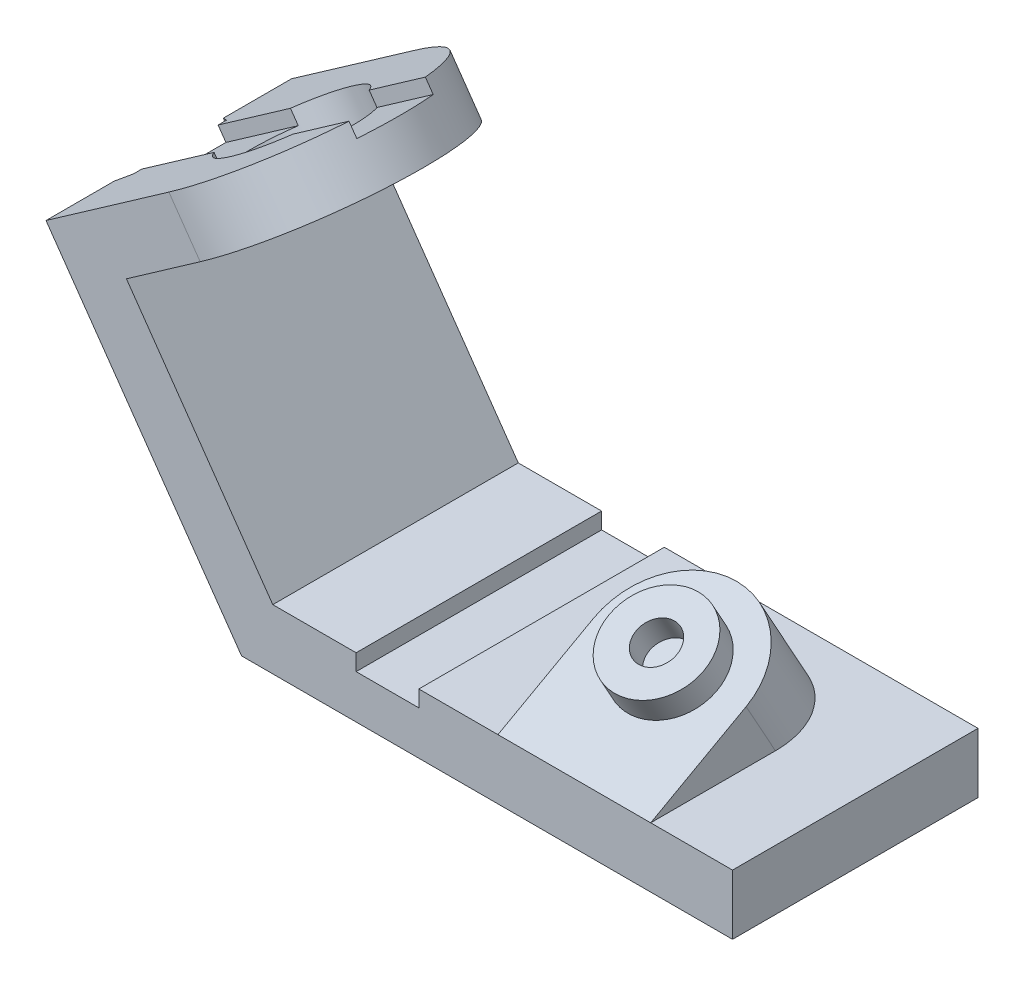
ISO-10303-21;
HEADER;
FILE_DESCRIPTION(('STEP AP214'),'2;1');
FILE_NAME('part.step','',(''),(''),'','','');
FILE_SCHEMA(('AUTOMOTIVE_DESIGN { 1 0 10303 214 1 1 1 1 }'));
ENDSEC;
DATA;
#1=APPLICATION_CONTEXT('core data for automotive mechanical design processes');
#2=APPLICATION_PROTOCOL_DEFINITION('international standard','automotive_design',2000,#1);
#3=PRODUCT_CONTEXT('',#1,'mechanical');
#4=PRODUCT('Part','Part','',(#3));
#5=PRODUCT_RELATED_PRODUCT_CATEGORY('part','',(#4));
#6=PRODUCT_DEFINITION_FORMATION('','',#4);
#7=PRODUCT_DEFINITION_CONTEXT('part definition',#1,'design');
#8=PRODUCT_DEFINITION('design','',#6,#7);
#9=PRODUCT_DEFINITION_SHAPE('','',#8);
#10=(LENGTH_UNIT() NAMED_UNIT(*) SI_UNIT(.MILLI.,.METRE.));
#11=(NAMED_UNIT(*) PLANE_ANGLE_UNIT() SI_UNIT($,.RADIAN.));
#12=(NAMED_UNIT(*) SI_UNIT($,.STERADIAN.) SOLID_ANGLE_UNIT());
#13=UNCERTAINTY_MEASURE_WITH_UNIT(LENGTH_MEASURE(1.E-05),#10,'distance_accuracy_value','');
#14=(GEOMETRIC_REPRESENTATION_CONTEXT(3) GLOBAL_UNCERTAINTY_ASSIGNED_CONTEXT((#13)) GLOBAL_UNIT_ASSIGNED_CONTEXT((#10,
#11,#12)) REPRESENTATION_CONTEXT('',''));
#15=CARTESIAN_POINT('',(0.,0.,0.));
#16=DIRECTION('',(0.,0.,1.));
#17=DIRECTION('',(1.,0.,0.));
#18=AXIS2_PLACEMENT_3D('',#15,#16,#17);
#19=CARTESIAN_POINT('',(-143.675709569523,115.012687135847,45.));
#20=DIRECTION('',(0.573576436351044,-0.819152044288993,0.));
#21=DIRECTION('',(0.819152044288993,0.573576436351044,0.));
#22=AXIS2_PLACEMENT_3D('',#19,#20,#21);
#23=PLANE('',#22);
#24=DIRECTION('',(0.,0.,-1.));
#25=VECTOR('',#24,1.);
#26=CARTESIAN_POINT('',(-157.601294322436,105.261887717879,-17.1132486540519));
#27=LINE('',#26,#25);
#28=CARTESIAN_POINT('',(-157.601294322436,105.261887717879,-14.));
#29=VERTEX_POINT('',#28);
#30=CARTESIAN_POINT('',(-157.601294322436,105.261887717879,-17.1132486540519));
#31=VERTEX_POINT('',#30);
#32=EDGE_CURVE('E277',#29,#31,#27,.T.);
#33=ORIENTED_EDGE('',*,*,#32,.F.);
#34=DIRECTION('',(-0.819152044288993,-0.573576436351044,0.));
#35=VECTOR('',#34,1.);
#36=CARTESIAN_POINT('',(-157.601294322436,105.261887717879,-14.));
#37=LINE('',#36,#35);
#38=CARTESIAN_POINT('',(-131.072166550331,123.837782966036,-14.));
#39=VERTEX_POINT('',#38);
#40=EDGE_CURVE('E236',#39,#29,#37,.T.);
#41=ORIENTED_EDGE('',*,*,#40,.F.);
#42=CARTESIAN_POINT('',(-116.643692107986,133.940709535432,0.));
#43=DIRECTION('',(-0.573576436351044,0.819152044288993,0.));
#44=DIRECTION('',(-0.819152044288993,-0.573576436351044,0.));
#45=AXIS2_PLACEMENT_3D('',#42,#43,#44);
#46=CIRCLE('',#45,22.5);
#47=CARTESIAN_POINT('',(-102.215217665641,144.043636104827,-14.));
#48=VERTEX_POINT('',#47);
#49=EDGE_CURVE('E292',#48,#39,#46,.T.);
#50=ORIENTED_EDGE('',*,*,#49,.F.);
#51=DIRECTION('',(-0.819152044288993,-0.573576436351044,0.));
#52=VECTOR('',#51,1.);
#53=CARTESIAN_POINT('',(-102.215217665641,144.043636104827,-14.));
#54=LINE('',#53,#52);
#55=CARTESIAN_POINT('',(-81.6111726286317,158.470743757354,-14.));
#56=VERTEX_POINT('',#55);
#57=EDGE_CURVE('E255',#56,#48,#54,.T.);
#58=ORIENTED_EDGE('',*,*,#57,.F.);
#59=CARTESIAN_POINT('',(-116.643692107986,133.940709535432,0.));
#60=DIRECTION('',(-0.573576436351044,0.819152044288993,0.));
#61=DIRECTION('',(-0.819152044288993,-0.573576436351044,0.));
#62=AXIS2_PLACEMENT_3D('',#59,#60,#61);
#63=CIRCLE('',#62,45.);
#64=CARTESIAN_POINT('',(-116.643692107986,133.940709535432,-45.));
#65=VERTEX_POINT('',#64);
#66=EDGE_CURVE('E314',#56,#65,#63,.T.);
#67=ORIENTED_EDGE('',*,*,#66,.T.);
#68=DIRECTION('',(-0.819152044288993,-0.573576436351044,0.));
#69=VECTOR('',#68,1.);
#70=CARTESIAN_POINT('',(-143.675709569523,115.012687135847,-45.));
#71=LINE('',#70,#69);
#72=CARTESIAN_POINT('',(-161.697054543881,102.394005536124,-45.));
#73=VERTEX_POINT('',#72);
#74=EDGE_CURVE('E336',#65,#73,#71,.T.);
#75=ORIENTED_EDGE('',*,*,#74,.T.);
#76=DIRECTION('',(0.,0.,1.));
#77=VECTOR('',#76,1.);
#78=CARTESIAN_POINT('',(-161.697054543881,102.394005536124,45.));
#79=LINE('',#78,#77);
#80=CARTESIAN_POINT('',(-161.697054543881,102.394005536124,-20.));
#81=VERTEX_POINT('',#80);
#82=EDGE_CURVE('E330',#73,#81,#79,.T.);
#83=ORIENTED_EDGE('',*,*,#82,.T.);
#84=DIRECTION('',(-0.709406479916225,-0.49673176489215,-0.500000000000001));
#85=VECTOR('',#84,1.);
#86=CARTESIAN_POINT('',(-161.697054543881,102.394005536124,-20.));
#87=LINE('',#86,#85);
#88=EDGE_CURVE('E279',#31,#81,#87,.T.);
#89=ORIENTED_EDGE('',*,*,#88,.F.);
#90=EDGE_LOOP('',(#33,#41,#50,#58,#67,#75,#83,#89));
#91=FACE_BOUND('',#90,.T.);
#92=ADVANCED_FACE('F44',(#91),#23,.F.);
#93=CARTESIAN_POINT('',(-60.3909064496553,-42.2861679353658,0.));
#94=DIRECTION('',(-0.819152044288993,-0.573576436351044,0.));
#95=DIRECTION('',(0.573576436351044,-0.819152044288993,0.));
#96=AXIS2_PLACEMENT_3D('',#93,#94,#95);
#97=PLANE('',#96);
#98=DIRECTION('',(0.573576436351044,-0.819152044288993,0.));
#99=VECTOR('',#98,1.);
#100=CARTESIAN_POINT('',(-60.3909064496553,-42.2861679353658,-20.));
#101=LINE('',#100,#99);
#102=CARTESIAN_POINT('',(-90.,0.,-20.));
#103=VERTEX_POINT('',#102);
#104=EDGE_CURVE('E52',#81,#103,#101,.T.);
#105=ORIENTED_EDGE('',*,*,#104,.F.);
#106=ORIENTED_EDGE('',*,*,#82,.F.);
#107=DIRECTION('',(-0.573576436351044,0.819152044288993,0.));
#108=VECTOR('',#107,1.);
#109=CARTESIAN_POINT('',(-90.,0.,-45.));
#110=LINE('',#109,#108);
#111=CARTESIAN_POINT('',(-90.,0.,-45.));
#112=VERTEX_POINT('',#111);
#113=EDGE_CURVE('E335',#112,#73,#110,.T.);
#114=ORIENTED_EDGE('',*,*,#113,.F.);
#115=DIRECTION('',(0.,0.,1.));
#116=VECTOR('',#115,1.);
#117=CARTESIAN_POINT('',(-90.,0.,45.));
#118=LINE('',#117,#116);
#119=EDGE_CURVE('E422',#112,#103,#118,.T.);
#120=ORIENTED_EDGE('',*,*,#119,.T.);
#121=EDGE_LOOP('',(#105,#106,#114,#120));
#122=FACE_BOUND('',#121,.T.);
#123=ADVANCED_FACE('F454',(#122),#97,.T.);
#124=CARTESIAN_POINT('',(-42.3695614752975,-29.6674863356428,0.));
#125=DIRECTION('',(-0.819152044288993,-0.573576436351044,0.));
#126=DIRECTION('',(0.573576436351044,-0.819152044288993,0.));
#127=AXIS2_PLACEMENT_3D('',#124,#125,#126);
#128=PLANE('',#127);
#129=DIRECTION('',(0.,0.,-1.));
#130=VECTOR('',#129,1.);
#131=CARTESIAN_POINT('',(-132.204180842502,98.6296462500672,0.));
#132=LINE('',#131,#130);
#133=CARTESIAN_POINT('',(-132.204180842502,98.6296462500672,45.));
#134=VERTEX_POINT('',#133);
#135=CARTESIAN_POINT('',(-132.204180842502,98.6296462500672,-45.));
#136=VERTEX_POINT('',#135);
#137=EDGE_CURVE('E318',#134,#136,#132,.T.);
#138=ORIENTED_EDGE('',*,*,#137,.F.);
#139=DIRECTION('',(0.573576436351044,-0.819152044288993,0.));
#140=VECTOR('',#139,1.);
#141=CARTESIAN_POINT('',(-71.9786550256421,12.618681599723,45.));
#142=LINE('',#141,#140);
#143=CARTESIAN_POINT('',(-78.5475248878616,22.,45.));
#144=VERTEX_POINT('',#143);
#145=EDGE_CURVE('E322',#134,#144,#142,.T.);
#146=ORIENTED_EDGE('',*,*,#145,.T.);
#147=DIRECTION('',(0.,0.,-1.));
#148=VECTOR('',#147,1.);
#149=CARTESIAN_POINT('',(-78.5475248878616,22.,0.));
#150=LINE('',#149,#148);
#151=CARTESIAN_POINT('',(-78.5475248878616,22.,-45.));
#152=VERTEX_POINT('',#151);
#153=EDGE_CURVE('E345',#144,#152,#150,.T.);
#154=ORIENTED_EDGE('',*,*,#153,.T.);
#155=DIRECTION('',(-0.573576436351044,0.819152044288993,0.));
#156=VECTOR('',#155,1.);
#157=CARTESIAN_POINT('',(-71.9786550256421,12.618681599723,-45.));
#158=LINE('',#157,#156);
#159=EDGE_CURVE('E326',#152,#136,#158,.T.);
#160=ORIENTED_EDGE('',*,*,#159,.T.);
#161=EDGE_LOOP('',(#138,#146,#154,#160));
#162=FACE_BOUND('',#161,.T.);
#163=ADVANCED_FACE('F474',(#162),#128,.F.);
#164=CARTESIAN_POINT('',(0.,22.,0.));
#165=DIRECTION('',(0.,-1.,0.));
#166=DIRECTION('',(0.,0.,-1.));
#167=AXIS2_PLACEMENT_3D('',#164,#165,#166);
#168=PLANE('',#167);
#169=ORIENTED_EDGE('',*,*,#153,.F.);
#170=DIRECTION('',(1.,0.,0.));
#171=VECTOR('',#170,1.);
#172=CARTESIAN_POINT('',(-90.,22.,45.));
#173=LINE('',#172,#171);
#174=CARTESIAN_POINT('',(-48.,22.,45.));
#175=VERTEX_POINT('',#174);
#176=EDGE_CURVE('E418',#144,#175,#173,.T.);
#177=ORIENTED_EDGE('',*,*,#176,.T.);
#178=DIRECTION('',(0.,0.,1.));
#179=VECTOR('',#178,1.);
#180=CARTESIAN_POINT('',(-48.,22.,-45.));
#181=LINE('',#180,#179);
#182=CARTESIAN_POINT('',(-48.,22.,-45.));
#183=VERTEX_POINT('',#182);
#184=EDGE_CURVE('E341',#183,#175,#181,.T.);
#185=ORIENTED_EDGE('',*,*,#184,.F.);
#186=DIRECTION('',(-1.,0.,0.));
#187=VECTOR('',#186,1.);
#188=CARTESIAN_POINT('',(-90.,22.,-45.));
#189=LINE('',#188,#187);
#190=EDGE_CURVE('E408',#183,#152,#189,.T.);
#191=ORIENTED_EDGE('',*,*,#190,.T.);
#192=EDGE_LOOP('',(#169,#177,#185,#191));
#193=FACE_BOUND('',#192,.T.);
#194=ADVANCED_FACE('F483',(#193),#168,.F.);
#195=CARTESIAN_POINT('',(90.,22.,45.));
#196=DIRECTION('',(-1.,0.,0.));
#197=DIRECTION('',(0.,0.,1.));
#198=AXIS2_PLACEMENT_3D('',#195,#196,#197);
#199=PLANE('',#198);
#200=DIRECTION('',(0.,0.,-1.));
#201=VECTOR('',#200,1.);
#202=CARTESIAN_POINT('',(90.,0.,45.));
#203=LINE('',#202,#201);
#204=CARTESIAN_POINT('',(90.,0.,45.));
#205=VERTEX_POINT('',#204);
#206=CARTESIAN_POINT('',(90.,0.,-45.));
#207=VERTEX_POINT('',#206);
#208=EDGE_CURVE('E394',#205,#207,#203,.T.);
#209=ORIENTED_EDGE('',*,*,#208,.T.);
#210=DIRECTION('',(0.,-1.,0.));
#211=VECTOR('',#210,1.);
#212=CARTESIAN_POINT('',(90.,22.,-45.));
#213=LINE('',#212,#211);
#214=CARTESIAN_POINT('',(90.,22.,-45.));
#215=VERTEX_POINT('',#214);
#216=EDGE_CURVE('E431',#215,#207,#213,.T.);
#217=ORIENTED_EDGE('',*,*,#216,.F.);
#218=DIRECTION('',(0.,0.,-1.));
#219=VECTOR('',#218,1.);
#220=CARTESIAN_POINT('',(90.,22.,45.));
#221=LINE('',#220,#219);
#222=CARTESIAN_POINT('',(90.,22.,45.));
#223=VERTEX_POINT('',#222);
#224=EDGE_CURVE('E409',#223,#215,#221,.T.);
#225=ORIENTED_EDGE('',*,*,#224,.F.);
#226=DIRECTION('',(0.,-1.,0.));
#227=VECTOR('',#226,1.);
#228=CARTESIAN_POINT('',(90.,22.,45.));
#229=LINE('',#228,#227);
#230=EDGE_CURVE('E416',#223,#205,#229,.T.);
#231=ORIENTED_EDGE('',*,*,#230,.T.);
#232=EDGE_LOOP('',(#209,#217,#225,#231));
#233=FACE_BOUND('',#232,.T.);
#234=ADVANCED_FACE('F50',(#233),#199,.F.);
#235=CARTESIAN_POINT('',(-90.,22.,-45.));
#236=DIRECTION('',(0.,0.,1.));
#237=DIRECTION('',(1.,0.,0.));
#238=AXIS2_PLACEMENT_3D('',#235,#236,#237);
#239=PLANE('',#238);
#240=ORIENTED_EDGE('',*,*,#74,.F.);
#241=DIRECTION('',(-0.573576436351044,0.819152044288993,0.));
#242=VECTOR('',#241,1.);
#243=CARTESIAN_POINT('',(-105.172163380965,117.557668649652,-45.));
#244=LINE('',#243,#242);
#245=CARTESIAN_POINT('',(-105.172163380965,117.557668649652,-45.));
#246=VERTEX_POINT('',#245);
#247=EDGE_CURVE('E313',#246,#65,#244,.T.);
#248=ORIENTED_EDGE('',*,*,#247,.F.);
#249=DIRECTION('',(-0.819152044288993,-0.573576436351044,0.));
#250=VECTOR('',#249,1.);
#251=CARTESIAN_POINT('',(-105.172163380965,117.557668649652,-45.));
#252=LINE('',#251,#250);
#253=EDGE_CURVE('E301',#246,#136,#252,.T.);
#254=ORIENTED_EDGE('',*,*,#253,.T.);
#255=ORIENTED_EDGE('',*,*,#159,.F.);
#256=ORIENTED_EDGE('',*,*,#190,.F.);
#257=DIRECTION('',(0.,1.,0.));
#258=VECTOR('',#257,1.);
#259=CARTESIAN_POINT('',(-48.,16.,-45.));
#260=LINE('',#259,#258);
#261=CARTESIAN_POINT('',(-48.,16.,-45.));
#262=VERTEX_POINT('',#261);
#263=EDGE_CURVE('E361',#262,#183,#260,.T.);
#264=ORIENTED_EDGE('',*,*,#263,.F.);
#265=DIRECTION('',(-1.,0.,0.));
#266=VECTOR('',#265,1.);
#267=CARTESIAN_POINT('',(-48.,16.,-45.));
#268=LINE('',#267,#266);
#269=CARTESIAN_POINT('',(-25.,16.,-45.));
#270=VERTEX_POINT('',#269);
#271=EDGE_CURVE('E357',#270,#262,#268,.T.);
#272=ORIENTED_EDGE('',*,*,#271,.F.);
#273=DIRECTION('',(0.,1.,0.));
#274=VECTOR('',#273,1.);
#275=CARTESIAN_POINT('',(-25.,16.,-45.));
#276=LINE('',#275,#274);
#277=CARTESIAN_POINT('',(-25.,22.,-45.));
#278=VERTEX_POINT('',#277);
#279=EDGE_CURVE('E368',#270,#278,#276,.T.);
#280=ORIENTED_EDGE('',*,*,#279,.T.);
#281=EDGE_CURVE('E415',#215,#278,#189,.T.);
#282=ORIENTED_EDGE('',*,*,#281,.F.);
#283=ORIENTED_EDGE('',*,*,#216,.T.);
#284=DIRECTION('',(-1.,0.,0.));
#285=VECTOR('',#284,1.);
#286=CARTESIAN_POINT('',(-90.,0.,-45.));
#287=LINE('',#286,#285);
#288=EDGE_CURVE('E425',#207,#112,#287,.T.);
#289=ORIENTED_EDGE('',*,*,#288,.T.);
#290=ORIENTED_EDGE('',*,*,#113,.T.);
#291=EDGE_LOOP('',(#240,#248,#254,#255,#256,#264,#272,#280,#282,#283,#289,#290));
#292=FACE_BOUND('',#291,.T.);
#293=ADVANCED_FACE('F460',(#292),#239,.F.);
#294=CARTESIAN_POINT('',(-90.,22.,45.));
#295=DIRECTION('',(0.,0.,-1.));
#296=DIRECTION('',(-1.,0.,0.));
#297=AXIS2_PLACEMENT_3D('',#294,#295,#296);
#298=PLANE('',#297);
#299=DIRECTION('',(0.573576436351044,-0.819152044288993,0.));
#300=VECTOR('',#299,1.);
#301=CARTESIAN_POINT('',(-90.,0.,45.));
#302=LINE('',#301,#300);
#303=CARTESIAN_POINT('',(-161.697054543881,102.394005536124,45.));
#304=VERTEX_POINT('',#303);
#305=CARTESIAN_POINT('',(-90.,0.,45.));
#306=VERTEX_POINT('',#305);
#307=EDGE_CURVE('E323',#304,#306,#302,.T.);
#308=ORIENTED_EDGE('',*,*,#307,.T.);
#309=DIRECTION('',(1.,0.,0.));
#310=VECTOR('',#309,1.);
#311=CARTESIAN_POINT('',(-90.,0.,45.));
#312=LINE('',#311,#310);
#313=EDGE_CURVE('E412',#306,#205,#312,.T.);
#314=ORIENTED_EDGE('',*,*,#313,.T.);
#315=ORIENTED_EDGE('',*,*,#230,.F.);
#316=CARTESIAN_POINT('',(60.,22.,45.));
#317=VERTEX_POINT('',#316);
#318=EDGE_CURVE('E411',#317,#223,#173,.T.);
#319=ORIENTED_EDGE('',*,*,#318,.F.);
#320=DIRECTION('',(-1.,0.,0.));
#321=VECTOR('',#320,1.);
#322=CARTESIAN_POINT('',(3.99999999999999,22.,45.));
#323=LINE('',#322,#321);
#324=CARTESIAN_POINT('',(3.99999999999999,22.,45.));
#325=VERTEX_POINT('',#324);
#326=EDGE_CURVE('E381',#317,#325,#323,.T.);
#327=ORIENTED_EDGE('',*,*,#326,.T.);
#328=CARTESIAN_POINT('',(-25.0000000000001,22.,45.));
#329=VERTEX_POINT('',#328);
#330=EDGE_CURVE('E420',#329,#325,#173,.T.);
#331=ORIENTED_EDGE('',*,*,#330,.F.);
#332=DIRECTION('',(0.,1.,0.));
#333=VECTOR('',#332,1.);
#334=CARTESIAN_POINT('',(-25.,16.,45.));
#335=LINE('',#334,#333);
#336=CARTESIAN_POINT('',(-25.,16.,45.));
#337=VERTEX_POINT('',#336);
#338=EDGE_CURVE('E369',#337,#329,#335,.T.);
#339=ORIENTED_EDGE('',*,*,#338,.F.);
#340=DIRECTION('',(1.,0.,0.));
#341=VECTOR('',#340,1.);
#342=CARTESIAN_POINT('',(-48.,16.,45.));
#343=LINE('',#342,#341);
#344=CARTESIAN_POINT('',(-48.,16.,45.));
#345=VERTEX_POINT('',#344);
#346=EDGE_CURVE('E349',#345,#337,#343,.T.);
#347=ORIENTED_EDGE('',*,*,#346,.F.);
#348=DIRECTION('',(0.,1.,0.));
#349=VECTOR('',#348,1.);
#350=CARTESIAN_POINT('',(-48.,16.,45.));
#351=LINE('',#350,#349);
#352=EDGE_CURVE('E359',#345,#175,#351,.T.);
#353=ORIENTED_EDGE('',*,*,#352,.T.);
#354=ORIENTED_EDGE('',*,*,#176,.F.);
#355=ORIENTED_EDGE('',*,*,#145,.F.);
#356=DIRECTION('',(0.819152044288993,0.573576436351044,0.));
#357=VECTOR('',#356,1.);
#358=CARTESIAN_POINT('',(-150.22552581686,86.0109646503443,45.));
#359=LINE('',#358,#357);
#360=CARTESIAN_POINT('',(-105.172163380965,117.557668649652,45.));
#361=VERTEX_POINT('',#360);
#362=EDGE_CURVE('E310',#134,#361,#359,.T.);
#363=ORIENTED_EDGE('',*,*,#362,.T.);
#364=DIRECTION('',(-0.573576436351044,0.819152044288993,0.));
#365=VECTOR('',#364,1.);
#366=CARTESIAN_POINT('',(-105.172163380965,117.557668649652,45.));
#367=LINE('',#366,#365);
#368=CARTESIAN_POINT('',(-116.643692107986,133.940709535432,45.));
#369=VERTEX_POINT('',#368);
#370=EDGE_CURVE('E312',#361,#369,#367,.T.);
#371=ORIENTED_EDGE('',*,*,#370,.T.);
#372=DIRECTION('',(-0.819152044288993,-0.573576436351044,0.));
#373=VECTOR('',#372,1.);
#374=CARTESIAN_POINT('',(-143.675709569523,115.012687135847,45.));
#375=LINE('',#374,#373);
#376=EDGE_CURVE('E328',#369,#304,#375,.T.);
#377=ORIENTED_EDGE('',*,*,#376,.T.);
#378=EDGE_LOOP('',(#308,#314,#315,#319,#327,#331,#339,#347,#353,#354,#355,#363,#371,#377));
#379=FACE_BOUND('',#378,.T.);
#380=ADVANCED_FACE('F479',(#379),#298,.F.);
#381=ORIENTED_EDGE('',*,*,#281,.T.);
#382=DIRECTION('',(0.,0.,-1.));
#383=VECTOR('',#382,1.);
#384=CARTESIAN_POINT('',(-25.,22.,-45.));
#385=LINE('',#384,#383);
#386=EDGE_CURVE('E348',#329,#278,#385,.T.);
#387=ORIENTED_EDGE('',*,*,#386,.F.);
#388=ORIENTED_EDGE('',*,*,#330,.T.);
#389=DIRECTION('',(0.,0.,-1.));
#390=VECTOR('',#389,1.);
#391=CARTESIAN_POINT('',(4.00000000000001,22.,-20.4679200720429));
#392=LINE('',#391,#390);
#393=CARTESIAN_POINT('',(4.,22.,-0.734162714932849));
#394=VERTEX_POINT('',#393);
#395=EDGE_CURVE('E405',#325,#394,#392,.T.);
#396=ORIENTED_EDGE('',*,*,#395,.T.);
#397=CARTESIAN_POINT('',(32.,22.,-0.734162714932849));
#398=DIRECTION('',(0.,-1.,0.));
#399=DIRECTION('',(0.,0.,1.));
#400=AXIS2_PLACEMENT_3D('',#397,#398,#399);
#401=ELLIPSE('',#400,32.013913900453,28.);
#402=CARTESIAN_POINT('',(60.,22.,-0.734162714932849));
#403=VERTEX_POINT('',#402);
#404=EDGE_CURVE('E393',#394,#403,#401,.T.);
#405=ORIENTED_EDGE('',*,*,#404,.T.);
#406=DIRECTION('',(0.,0.,1.));
#407=VECTOR('',#406,1.);
#408=CARTESIAN_POINT('',(60.,22.,14.5168682135329));
#409=LINE('',#408,#407);
#410=EDGE_CURVE('E399',#403,#317,#409,.T.);
#411=ORIENTED_EDGE('',*,*,#410,.T.);
#412=ORIENTED_EDGE('',*,*,#318,.T.);
#413=ORIENTED_EDGE('',*,*,#224,.T.);
#414=EDGE_LOOP('',(#381,#387,#388,#396,#405,#411,#412,#413));
#415=FACE_BOUND('',#414,.T.);
#416=ADVANCED_FACE('F500',(#415),#168,.F.);
#417=CARTESIAN_POINT('',(0.,0.,0.));
#418=DIRECTION('',(0.,-1.,0.));
#419=DIRECTION('',(0.,0.,-1.));
#420=AXIS2_PLACEMENT_3D('',#417,#418,#419);
#421=PLANE('',#420);
#422=DIRECTION('',(0.903998769549426,0.,0.427535056636439));
#423=VECTOR('',#422,1.);
#424=CARTESIAN_POINT('',(-8.72093691600937,0.,18.4399293555351));
#425=LINE('',#424,#423);
#426=CARTESIAN_POINT('',(-83.8961270561927,0.,-17.1132486540519));
#427=VERTEX_POINT('',#426);
#428=EDGE_CURVE('E290',#103,#427,#425,.T.);
#429=ORIENTED_EDGE('',*,*,#428,.F.);
#430=ORIENTED_EDGE('',*,*,#119,.F.);
#431=ORIENTED_EDGE('',*,*,#288,.F.);
#432=ORIENTED_EDGE('',*,*,#208,.F.);
#433=ORIENTED_EDGE('',*,*,#313,.F.);
#434=CARTESIAN_POINT('',(-90.,0.,20.));
#435=VERTEX_POINT('',#434);
#436=EDGE_CURVE('E424',#435,#306,#118,.T.);
#437=ORIENTED_EDGE('',*,*,#436,.F.);
#438=DIRECTION('',(-0.903998769549427,0.,0.427535056636438));
#439=VECTOR('',#438,1.);
#440=CARTESIAN_POINT('',(-8.7209369160093,0.,-18.439929355535));
#441=LINE('',#440,#439);
#442=CARTESIAN_POINT('',(-83.8961270561927,0.,17.1132486540519));
#443=VERTEX_POINT('',#442);
#444=EDGE_CURVE('E281',#443,#435,#441,.T.);
#445=ORIENTED_EDGE('',*,*,#444,.F.);
#446=DIRECTION('',(0.,0.,1.));
#447=VECTOR('',#446,1.);
#448=CARTESIAN_POINT('',(-83.8961270561927,0.,0.));
#449=LINE('',#448,#447);
#450=EDGE_CURVE('E289',#427,#443,#449,.T.);
#451=ORIENTED_EDGE('',*,*,#450,.F.);
#452=EDGE_LOOP('',(#429,#430,#431,#432,#433,#437,#445,#451));
#453=FACE_BOUND('',#452,.T.);
#454=ADVANCED_FACE('F452',(#453),#421,.T.);
#455=CARTESIAN_POINT('',(60.,-32.9930254730188,14.5168682135329));
#456=DIRECTION('',(-1.,0.,0.));
#457=DIRECTION('',(0.,0.,1.));
#458=AXIS2_PLACEMENT_3D('',#455,#456,#457);
#459=PLANE('',#458);
#460=ORIENTED_EDGE('',*,*,#410,.F.);
#461=DIRECTION('',(0.,0.874619707139395,0.484809620246339));
#462=VECTOR('',#461,1.);
#463=CARTESIAN_POINT('',(60.,-13.6006406631652,-20.4679200720429));
#464=LINE('',#463,#462);
#465=CARTESIAN_POINT('',(60.,41.3923848098536,10.0152117144242));
#466=VERTEX_POINT('',#465);
#467=EDGE_CURVE('E395',#403,#466,#464,.T.);
#468=ORIENTED_EDGE('',*,*,#467,.T.);
#469=DIRECTION('',(0.,-0.484809620246339,0.874619707139395));
#470=VECTOR('',#469,1.);
#471=CARTESIAN_POINT('',(60.,22.,45.));
#472=LINE('',#471,#470);
#473=EDGE_CURVE('E385',#466,#317,#472,.T.);
#474=ORIENTED_EDGE('',*,*,#473,.T.);
#475=EDGE_LOOP('',(#460,#468,#474));
#476=FACE_BOUND('',#475,.T.);
#477=ADVANCED_FACE('F576',(#476),#459,.F.);
#478=CARTESIAN_POINT('',(4.,-13.6006406631652,-20.4679200720429));
#479=DIRECTION('',(1.,0.,0.));
#480=DIRECTION('',(0.,0.,-1.));
#481=AXIS2_PLACEMENT_3D('',#478,#479,#480);
#482=PLANE('',#481);
#483=ORIENTED_EDGE('',*,*,#395,.F.);
#484=DIRECTION('',(0.,0.484809620246339,-0.874619707139395));
#485=VECTOR('',#484,1.);
#486=CARTESIAN_POINT('',(4.,41.3923848098536,10.0152117144242));
#487=LINE('',#486,#485);
#488=CARTESIAN_POINT('',(4.,41.3923848098536,10.0152117144242));
#489=VERTEX_POINT('',#488);
#490=EDGE_CURVE('E387',#325,#489,#487,.T.);
#491=ORIENTED_EDGE('',*,*,#490,.T.);
#492=DIRECTION('',(0.,0.874619707139395,0.484809620246339));
#493=VECTOR('',#492,1.);
#494=CARTESIAN_POINT('',(4.,-13.6006406631652,-20.4679200720429));
#495=LINE('',#494,#493);
#496=EDGE_CURVE('E386',#394,#489,#495,.T.);
#497=ORIENTED_EDGE('',*,*,#496,.F.);
#498=EDGE_LOOP('',(#483,#491,#497));
#499=FACE_BOUND('',#498,.T.);
#500=ADVANCED_FACE('F587',(#499),#482,.F.);
#501=CARTESIAN_POINT('',(32.,-13.6006406631652,-20.4679200720429));
#502=DIRECTION('',(0.,0.874619707139395,0.484809620246339));
#503=DIRECTION('',(0.,-0.484809620246339,0.874619707139395));
#504=AXIS2_PLACEMENT_3D('',#501,#502,#503);
#505=CYLINDRICAL_SURFACE('',#504,28.);
#506=ORIENTED_EDGE('',*,*,#404,.F.);
#507=ORIENTED_EDGE('',*,*,#496,.T.);
#508=CARTESIAN_POINT('',(32.,41.3923848098536,10.0152117144242));
#509=DIRECTION('',(0.,-0.874619707139395,-0.484809620246339));
#510=DIRECTION('',(0.,0.484809620246339,-0.874619707139395));
#511=AXIS2_PLACEMENT_3D('',#508,#509,#510);
#512=CIRCLE('',#511,28.);
#513=EDGE_CURVE('E384',#489,#466,#512,.T.);
#514=ORIENTED_EDGE('',*,*,#513,.T.);
#515=ORIENTED_EDGE('',*,*,#467,.F.);
#516=EDGE_LOOP('',(#506,#507,#514,#515));
#517=FACE_BOUND('',#516,.T.);
#518=ADVANCED_FACE('F588',(#517),#505,.T.);
#519=CARTESIAN_POINT('',(32.,41.3923848098536,10.0152117144242));
#520=DIRECTION('',(0.,-0.874619707139395,-0.484809620246339));
#521=DIRECTION('',(0.,0.484809620246339,-0.874619707139395));
#522=AXIS2_PLACEMENT_3D('',#519,#520,#521);
#523=PLANE('',#522);
#524=CARTESIAN_POINT('',(32.,41.3923848098536,10.0152117144242));
#525=DIRECTION('',(0.,-0.874619707139395,-0.484809620246339));
#526=DIRECTION('',(0.,0.484809620246339,-0.874619707139395));
#527=AXIS2_PLACEMENT_3D('',#524,#525,#526);
#528=CIRCLE('',#527,17.5);
#529=CARTESIAN_POINT('',(32.,49.8765531641645,-5.2906331605152));
#530=VERTEX_POINT('',#529);
#531=EDGE_CURVE('E432',#530,#530,#528,.F.);
#532=ORIENTED_EDGE('',*,*,#531,.F.);
#533=EDGE_LOOP('',(#532));
#534=FACE_BOUND('',#533,.T.);
#535=ORIENTED_EDGE('',*,*,#513,.F.);
#536=ORIENTED_EDGE('',*,*,#490,.F.);
#537=ORIENTED_EDGE('',*,*,#326,.F.);
#538=ORIENTED_EDGE('',*,*,#473,.F.);
#539=EDGE_LOOP('',(#535,#536,#537,#538));
#540=FACE_BOUND('',#539,.T.);
#541=ADVANCED_FACE('F578',(#534,#540),#523,.F.);
#542=CARTESIAN_POINT('',(32.,50.1385818812475,14.8633079168876));
#543=DIRECTION('',(0.,0.874619707139395,0.484809620246339));
#544=DIRECTION('',(0.,-0.484809620246339,0.874619707139395));
#545=AXIS2_PLACEMENT_3D('',#542,#543,#544);
#546=PLANE('',#545);
#547=CARTESIAN_POINT('',(32.,50.1385818812475,14.8633079168876));
#548=DIRECTION('',(0.,0.874619707139395,0.484809620246339));
#549=DIRECTION('',(0.,-0.484809620246339,0.874619707139395));
#550=AXIS2_PLACEMENT_3D('',#547,#548,#549);
#551=CIRCLE('',#550,17.5);
#552=CARTESIAN_POINT('',(32.,41.6544135269366,30.169152791827));
#553=VERTEX_POINT('',#552);
#554=EDGE_CURVE('E376',#553,#553,#551,.T.);
#555=ORIENTED_EDGE('',*,*,#554,.T.);
#556=EDGE_LOOP('',(#555));
#557=FACE_BOUND('',#556,.T.);
#558=CARTESIAN_POINT('',(32.,50.1385818812475,14.8633079168876));
#559=DIRECTION('',(0.,0.874619707139395,0.484809620246339));
#560=DIRECTION('',(0.,-0.484809620246339,0.874619707139395));
#561=AXIS2_PLACEMENT_3D('',#558,#559,#560);
#562=CIRCLE('',#561,7.5);
#563=CARTESIAN_POINT('',(32.,46.5025097294,21.4229557204331));
#564=VERTEX_POINT('',#563);
#565=EDGE_CURVE('E373',#564,#564,#562,.T.);
#566=ORIENTED_EDGE('',*,*,#565,.F.);
#567=EDGE_LOOP('',(#566));
#568=FACE_BOUND('',#567,.T.);
#569=ADVANCED_FACE('F573',(#557,#568),#546,.T.);
#570=CARTESIAN_POINT('',(32.,50.1385818812475,14.8633079168876));
#571=DIRECTION('',(0.,-0.874619707139395,-0.484809620246339));
#572=DIRECTION('',(0.,0.484809620246339,-0.874619707139395));
#573=AXIS2_PLACEMENT_3D('',#570,#571,#572);
#574=CYLINDRICAL_SURFACE('',#573,17.5);
#575=ORIENTED_EDGE('',*,*,#554,.F.);
#576=EDGE_LOOP('',(#575));
#577=FACE_BOUND('',#576,.T.);
#578=ORIENTED_EDGE('',*,*,#531,.T.);
#579=EDGE_LOOP('',(#578));
#580=FACE_BOUND('',#579,.T.);
#581=ADVANCED_FACE('F575',(#577,#580),#574,.T.);
#582=CARTESIAN_POINT('',(32.,50.1385818812475,14.8633079168876));
#583=DIRECTION('',(0.,-0.874619707139395,-0.484809620246339));
#584=DIRECTION('',(0.,0.484809620246339,-0.874619707139395));
#585=AXIS2_PLACEMENT_3D('',#582,#583,#584);
#586=CYLINDRICAL_SURFACE('',#585,7.5);
#587=ORIENTED_EDGE('',*,*,#565,.T.);
#588=EDGE_LOOP('',(#587));
#589=FACE_BOUND('',#588,.T.);
#590=CARTESIAN_POINT('',(32.,41.3923848098536,10.0152117144242));
#591=DIRECTION('',(0.,0.874619707139395,0.484809620246339));
#592=DIRECTION('',(0.,-0.484809620246339,0.874619707139395));
#593=AXIS2_PLACEMENT_3D('',#590,#591,#592);
#594=CIRCLE('',#593,7.5);
#595=CARTESIAN_POINT('',(32.,37.756312658006,16.5748595179697));
#596=VERTEX_POINT('',#595);
#597=EDGE_CURVE('E364',#596,#596,#594,.T.);
#598=ORIENTED_EDGE('',*,*,#597,.F.);
#599=EDGE_LOOP('',(#598));
#600=FACE_BOUND('',#599,.T.);
#601=ADVANCED_FACE('F568',(#589,#600),#586,.F.);
#602=ORIENTED_EDGE('',*,*,#597,.T.);
#603=EDGE_LOOP('',(#602));
#604=FACE_BOUND('',#603,.T.);
#605=ADVANCED_FACE('F569',(#604),#523,.F.);
#606=CARTESIAN_POINT('',(-48.,16.,-45.));
#607=DIRECTION('',(-1.,0.,0.));
#608=DIRECTION('',(0.,0.,1.));
#609=AXIS2_PLACEMENT_3D('',#606,#607,#608);
#610=PLANE('',#609);
#611=ORIENTED_EDGE('',*,*,#184,.T.);
#612=ORIENTED_EDGE('',*,*,#352,.F.);
#613=DIRECTION('',(0.,0.,1.));
#614=VECTOR('',#613,1.);
#615=CARTESIAN_POINT('',(-48.,16.,-45.));
#616=LINE('',#615,#614);
#617=EDGE_CURVE('E347',#262,#345,#616,.T.);
#618=ORIENTED_EDGE('',*,*,#617,.F.);
#619=ORIENTED_EDGE('',*,*,#263,.T.);
#620=EDGE_LOOP('',(#611,#612,#618,#619));
#621=FACE_BOUND('',#620,.T.);
#622=ADVANCED_FACE('F486',(#621),#610,.F.);
#623=CARTESIAN_POINT('',(-25.,16.,-45.));
#624=DIRECTION('',(1.,0.,0.));
#625=DIRECTION('',(0.,0.,-1.));
#626=AXIS2_PLACEMENT_3D('',#623,#624,#625);
#627=PLANE('',#626);
#628=ORIENTED_EDGE('',*,*,#386,.T.);
#629=ORIENTED_EDGE('',*,*,#279,.F.);
#630=DIRECTION('',(0.,0.,-1.));
#631=VECTOR('',#630,1.);
#632=CARTESIAN_POINT('',(-25.,16.,-45.));
#633=LINE('',#632,#631);
#634=EDGE_CURVE('E355',#337,#270,#633,.T.);
#635=ORIENTED_EDGE('',*,*,#634,.F.);
#636=ORIENTED_EDGE('',*,*,#338,.T.);
#637=EDGE_LOOP('',(#628,#629,#635,#636));
#638=FACE_BOUND('',#637,.T.);
#639=ADVANCED_FACE('F492',(#638),#627,.F.);
#640=CARTESIAN_POINT('',(0.,16.,0.));
#641=DIRECTION('',(0.,1.,0.));
#642=DIRECTION('',(0.,0.,1.));
#643=AXIS2_PLACEMENT_3D('',#640,#641,#642);
#644=PLANE('',#643);
#645=ORIENTED_EDGE('',*,*,#617,.T.);
#646=ORIENTED_EDGE('',*,*,#346,.T.);
#647=ORIENTED_EDGE('',*,*,#634,.T.);
#648=ORIENTED_EDGE('',*,*,#271,.T.);
#649=EDGE_LOOP('',(#645,#646,#647,#648));
#650=FACE_BOUND('',#649,.T.);
#651=ADVANCED_FACE('F489',(#650),#644,.T.);
#652=CARTESIAN_POINT('',(-131.072166550331,123.837782966036,14.));
#653=VERTEX_POINT('',#652);
#654=CARTESIAN_POINT('',(-102.215217665641,144.043636104827,14.));
#655=VERTEX_POINT('',#654);
#656=EDGE_CURVE('E295',#653,#655,#46,.T.);
#657=ORIENTED_EDGE('',*,*,#656,.F.);
#658=DIRECTION('',(0.819152044288993,0.573576436351044,0.));
#659=VECTOR('',#658,1.);
#660=CARTESIAN_POINT('',(-157.601294322436,105.261887717879,14.));
#661=LINE('',#660,#659);
#662=CARTESIAN_POINT('',(-157.601294322436,105.261887717879,14.));
#663=VERTEX_POINT('',#662);
#664=EDGE_CURVE('E261',#663,#653,#661,.T.);
#665=ORIENTED_EDGE('',*,*,#664,.F.);
#666=CARTESIAN_POINT('',(-157.601294322436,105.261887717879,17.1132486540519));
#667=VERTEX_POINT('',#666);
#668=EDGE_CURVE('E245',#667,#663,#27,.T.);
#669=ORIENTED_EDGE('',*,*,#668,.F.);
#670=DIRECTION('',(0.709406479916225,0.49673176489215,-0.5));
#671=VECTOR('',#670,1.);
#672=CARTESIAN_POINT('',(-161.697054543881,102.394005536124,20.));
#673=LINE('',#672,#671);
#674=CARTESIAN_POINT('',(-161.697054543881,102.394005536124,20.));
#675=VERTEX_POINT('',#674);
#676=EDGE_CURVE('E272',#675,#667,#673,.T.);
#677=ORIENTED_EDGE('',*,*,#676,.F.);
#678=EDGE_CURVE('E331',#675,#304,#79,.T.);
#679=ORIENTED_EDGE('',*,*,#678,.T.);
#680=ORIENTED_EDGE('',*,*,#376,.F.);
#681=CARTESIAN_POINT('',(-81.6111726286317,158.470743757354,14.));
#682=VERTEX_POINT('',#681);
#683=EDGE_CURVE('E308',#369,#682,#63,.T.);
#684=ORIENTED_EDGE('',*,*,#683,.T.);
#685=DIRECTION('',(0.819152044288993,0.573576436351044,0.));
#686=VECTOR('',#685,1.);
#687=CARTESIAN_POINT('',(-102.215217665641,144.043636104827,14.));
#688=LINE('',#687,#686);
#689=EDGE_CURVE('E260',#655,#682,#688,.T.);
#690=ORIENTED_EDGE('',*,*,#689,.F.);
#691=EDGE_LOOP('',(#657,#665,#669,#677,#679,#680,#684,#690));
#692=FACE_BOUND('',#691,.T.);
#693=ADVANCED_FACE('F517',(#692),#23,.F.);
#694=DIRECTION('',(-0.573576436351044,0.819152044288993,0.));
#695=VECTOR('',#694,1.);
#696=CARTESIAN_POINT('',(-60.3909064496553,-42.2861679353658,20.));
#697=LINE('',#696,#695);
#698=EDGE_CURVE('E440',#435,#675,#697,.T.);
#699=ORIENTED_EDGE('',*,*,#698,.F.);
#700=ORIENTED_EDGE('',*,*,#436,.T.);
#701=ORIENTED_EDGE('',*,*,#307,.F.);
#702=ORIENTED_EDGE('',*,*,#678,.F.);
#703=EDGE_LOOP('',(#699,#700,#701,#702));
#704=FACE_BOUND('',#703,.T.);
#705=ADVANCED_FACE('F512',(#704),#97,.T.);
#706=CARTESIAN_POINT('',(-105.172163380965,117.557668649652,0.));
#707=DIRECTION('',(-0.573576436351044,0.819152044288993,0.));
#708=DIRECTION('',(-0.819152044288993,-0.573576436351044,0.));
#709=AXIS2_PLACEMENT_3D('',#706,#707,#708);
#710=PLANE('',#709);
#711=CARTESIAN_POINT('',(-105.172163380965,117.557668649652,0.));
#712=DIRECTION('',(-0.573576436351044,0.819152044288993,0.));
#713=DIRECTION('',(-0.819152044288993,-0.573576436351044,0.));
#714=AXIS2_PLACEMENT_3D('',#711,#712,#713);
#715=CIRCLE('',#714,11.);
#716=CARTESIAN_POINT('',(-114.182835868144,111.24832784979,0.));
#717=VERTEX_POINT('',#716);
#718=EDGE_CURVE('E302',#717,#717,#715,.T.);
#719=ORIENTED_EDGE('',*,*,#718,.T.);
#720=EDGE_LOOP('',(#719));
#721=FACE_BOUND('',#720,.T.);
#722=ORIENTED_EDGE('',*,*,#362,.F.);
#723=ORIENTED_EDGE('',*,*,#137,.T.);
#724=ORIENTED_EDGE('',*,*,#253,.F.);
#725=CARTESIAN_POINT('',(-105.172163380965,117.557668649652,0.));
#726=DIRECTION('',(-0.573576436351044,0.819152044288993,0.));
#727=DIRECTION('',(-0.819152044288993,-0.573576436351044,0.));
#728=AXIS2_PLACEMENT_3D('',#725,#726,#727);
#729=CIRCLE('',#728,45.);
#730=EDGE_CURVE('E305',#361,#246,#729,.T.);
#731=ORIENTED_EDGE('',*,*,#730,.F.);
#732=EDGE_LOOP('',(#722,#723,#724,#731));
#733=FACE_BOUND('',#732,.T.);
#734=ADVANCED_FACE('F472',(#721,#733),#710,.F.);
#735=CARTESIAN_POINT('',(-105.172163380965,117.557668649652,0.));
#736=DIRECTION('',(-0.573576436351044,0.819152044288993,0.));
#737=DIRECTION('',(-0.819152044288993,-0.573576436351044,0.));
#738=AXIS2_PLACEMENT_3D('',#735,#736,#737);
#739=CYLINDRICAL_SURFACE('',#738,45.);
#740=DIRECTION('',(-0.573576436351044,0.819152044288993,0.));
#741=VECTOR('',#740,1.);
#742=CARTESIAN_POINT('',(-70.1396439016108,142.087702871574,-14.));
#743=LINE('',#742,#741);
#744=CARTESIAN_POINT('',(-78.7432904468765,154.374983535909,-14.));
#745=VERTEX_POINT('',#744);
#746=EDGE_CURVE('E271',#745,#56,#743,.T.);
#747=ORIENTED_EDGE('',*,*,#746,.F.);
#748=CARTESIAN_POINT('',(-113.775809926231,129.844949313987,0.));
#749=DIRECTION('',(-0.573576436351044,0.819152044288993,0.));
#750=DIRECTION('',(-0.819152044288993,-0.573576436351044,0.));
#751=AXIS2_PLACEMENT_3D('',#748,#749,#750);
#752=CIRCLE('',#751,45.);
#753=CARTESIAN_POINT('',(-78.7432904468765,154.374983535909,14.));
#754=VERTEX_POINT('',#753);
#755=EDGE_CURVE('E264',#745,#754,#752,.F.);
#756=ORIENTED_EDGE('',*,*,#755,.T.);
#757=DIRECTION('',(-0.573576436351044,0.819152044288993,0.));
#758=VECTOR('',#757,1.);
#759=CARTESIAN_POINT('',(-70.1396439016108,142.087702871574,14.));
#760=LINE('',#759,#758);
#761=EDGE_CURVE('E267',#682,#754,#760,.F.);
#762=ORIENTED_EDGE('',*,*,#761,.F.);
#763=ORIENTED_EDGE('',*,*,#683,.F.);
#764=ORIENTED_EDGE('',*,*,#370,.F.);
#765=ORIENTED_EDGE('',*,*,#730,.T.);
#766=ORIENTED_EDGE('',*,*,#247,.T.);
#767=ORIENTED_EDGE('',*,*,#66,.F.);
#768=EDGE_LOOP('',(#747,#756,#762,#763,#764,#765,#766,#767));
#769=FACE_BOUND('',#768,.T.);
#770=ADVANCED_FACE('F463',(#769),#739,.T.);
#771=CARTESIAN_POINT('',(-116.643692107986,133.940709535432,0.));
#772=DIRECTION('',(-0.573576436351044,0.819152044288993,0.));
#773=DIRECTION('',(-0.819152044288993,-0.573576436351044,0.));
#774=AXIS2_PLACEMENT_3D('',#771,#772,#773);
#775=CYLINDRICAL_SURFACE('',#774,11.);
#776=CARTESIAN_POINT('',(-109.760774871773,124.110885003964,0.));
#777=DIRECTION('',(-0.573576436351044,0.819152044288993,0.));
#778=DIRECTION('',(-0.819152044288993,-0.573576436351044,0.));
#779=AXIS2_PLACEMENT_3D('',#776,#777,#778);
#780=CIRCLE('',#779,11.);
#781=CARTESIAN_POINT('',(-118.771447358952,117.801544204102,0.));
#782=VERTEX_POINT('',#781);
#783=EDGE_CURVE('E300',#782,#782,#780,.T.);
#784=ORIENTED_EDGE('',*,*,#783,.T.);
#785=EDGE_LOOP('',(#784));
#786=FACE_BOUND('',#785,.T.);
#787=ORIENTED_EDGE('',*,*,#718,.F.);
#788=EDGE_LOOP('',(#787));
#789=FACE_BOUND('',#788,.T.);
#790=ADVANCED_FACE('F619',(#786,#789),#775,.F.);
#791=CARTESIAN_POINT('',(-109.760774871773,124.110885003964,11.));
#792=DIRECTION('',(0.573576436351044,-0.819152044288993,0.));
#793=DIRECTION('',(0.819152044288993,0.573576436351044,0.));
#794=AXIS2_PLACEMENT_3D('',#791,#792,#793);
#795=PLANE('',#794);
#796=ORIENTED_EDGE('',*,*,#783,.F.);
#797=EDGE_LOOP('',(#796));
#798=FACE_BOUND('',#797,.T.);
#799=CARTESIAN_POINT('',(-109.760774871773,124.110885003964,0.));
#800=DIRECTION('',(-0.573576436351044,0.819152044288993,0.));
#801=DIRECTION('',(-0.819152044288993,-0.573576436351044,0.));
#802=AXIS2_PLACEMENT_3D('',#799,#800,#801);
#803=CIRCLE('',#802,22.5);
#804=CARTESIAN_POINT('',(-128.191695868276,111.205415186065,0.));
#805=VERTEX_POINT('',#804);
#806=EDGE_CURVE('E293',#805,#805,#803,.T.);
#807=ORIENTED_EDGE('',*,*,#806,.T.);
#808=EDGE_LOOP('',(#807));
#809=FACE_BOUND('',#808,.T.);
#810=ADVANCED_FACE('F624',(#798,#809),#795,.F.);
#811=CARTESIAN_POINT('',(-116.643692107986,133.940709535432,0.));
#812=DIRECTION('',(-0.573576436351044,0.819152044288993,0.));
#813=DIRECTION('',(-0.819152044288993,-0.573576436351044,0.));
#814=AXIS2_PLACEMENT_3D('',#811,#812,#813);
#815=CYLINDRICAL_SURFACE('',#814,22.5);
#816=ORIENTED_EDGE('',*,*,#49,.T.);
#817=DIRECTION('',(-0.573576436351044,0.819152044288993,0.));
#818=VECTOR('',#817,1.);
#819=CARTESIAN_POINT('',(-128.204284368575,119.742022744591,-14.));
#820=LINE('',#819,#818);
#821=CARTESIAN_POINT('',(-128.204284368575,119.742022744591,-14.));
#822=VERTEX_POINT('',#821);
#823=EDGE_CURVE('E243',#822,#39,#820,.T.);
#824=ORIENTED_EDGE('',*,*,#823,.F.);
#825=CARTESIAN_POINT('',(-113.775809926231,129.844949313987,0.));
#826=DIRECTION('',(-0.573576436351044,0.819152044288993,0.));
#827=DIRECTION('',(-0.819152044288993,-0.573576436351044,0.));
#828=AXIS2_PLACEMENT_3D('',#825,#826,#827);
#829=CIRCLE('',#828,22.5);
#830=CARTESIAN_POINT('',(-128.204284368575,119.742022744591,14.));
#831=VERTEX_POINT('',#830);
#832=EDGE_CURVE('E263',#831,#822,#829,.F.);
#833=ORIENTED_EDGE('',*,*,#832,.F.);
#834=DIRECTION('',(-0.573576436351044,0.819152044288993,0.));
#835=VECTOR('',#834,1.);
#836=CARTESIAN_POINT('',(-128.204284368575,119.742022744591,14.));
#837=LINE('',#836,#835);
#838=EDGE_CURVE('E228',#831,#653,#837,.T.);
#839=ORIENTED_EDGE('',*,*,#838,.T.);
#840=ORIENTED_EDGE('',*,*,#656,.T.);
#841=DIRECTION('',(-0.573576436351044,0.819152044288993,0.));
#842=VECTOR('',#841,1.);
#843=CARTESIAN_POINT('',(-99.3473354838859,139.947875883382,14.));
#844=LINE('',#843,#842);
#845=CARTESIAN_POINT('',(-99.3473354838859,139.947875883382,14.));
#846=VERTEX_POINT('',#845);
#847=EDGE_CURVE('E258',#846,#655,#844,.T.);
#848=ORIENTED_EDGE('',*,*,#847,.F.);
#849=CARTESIAN_POINT('',(-113.775809926231,129.844949313987,0.));
#850=DIRECTION('',(-0.573576436351044,0.819152044288993,0.));
#851=DIRECTION('',(-0.819152044288993,-0.573576436351044,0.));
#852=AXIS2_PLACEMENT_3D('',#849,#850,#851);
#853=CIRCLE('',#852,22.5);
#854=CARTESIAN_POINT('',(-99.3473354838859,139.947875883382,-14.));
#855=VERTEX_POINT('',#854);
#856=EDGE_CURVE('E11',#855,#846,#853,.F.);
#857=ORIENTED_EDGE('',*,*,#856,.F.);
#858=DIRECTION('',(-0.573576436351044,0.819152044288993,0.));
#859=VECTOR('',#858,1.);
#860=CARTESIAN_POINT('',(-99.3473354838859,139.947875883382,-14.));
#861=LINE('',#860,#859);
#862=EDGE_CURVE('E58',#855,#48,#861,.T.);
#863=ORIENTED_EDGE('',*,*,#862,.T.);
#864=EDGE_LOOP('',(#816,#824,#833,#839,#840,#848,#857,#863));
#865=FACE_BOUND('',#864,.T.);
#866=ORIENTED_EDGE('',*,*,#806,.F.);
#867=EDGE_LOOP('',(#866));
#868=FACE_BOUND('',#867,.T.);
#869=ADVANCED_FACE('F526',(#865,#868),#815,.F.);
#870=CARTESIAN_POINT('',(-30.7818128993106,-84.5723358707316,-20.));
#871=DIRECTION('',(0.409576022144498,0.286788218175523,-0.866025403784438));
#872=DIRECTION('',(-0.903998769549426,0.,-0.427535056636439));
#873=AXIS2_PLACEMENT_3D('',#870,#871,#872);
#874=PLANE('',#873);
#875=ORIENTED_EDGE('',*,*,#428,.T.);
#876=DIRECTION('',(-0.573576436351044,0.819152044288993,0.));
#877=VECTOR('',#876,1.);
#878=CARTESIAN_POINT('',(-26.6860526778656,-81.7044536889764,-17.1132486540519));
#879=LINE('',#878,#877);
#880=EDGE_CURVE('E282',#427,#31,#879,.T.);
#881=ORIENTED_EDGE('',*,*,#880,.T.);
#882=ORIENTED_EDGE('',*,*,#88,.T.);
#883=ORIENTED_EDGE('',*,*,#104,.T.);
#884=EDGE_LOOP('',(#875,#881,#882,#883));
#885=FACE_BOUND('',#884,.T.);
#886=ADVANCED_FACE('F444',(#885),#874,.F.);
#887=CARTESIAN_POINT('',(-26.6860526778656,-81.7044536889764,-17.1132486540519));
#888=DIRECTION('',(0.819152044288993,0.573576436351044,0.));
#889=DIRECTION('',(-0.573576436351044,0.819152044288993,0.));
#890=AXIS2_PLACEMENT_3D('',#887,#888,#889);
#891=PLANE('',#890);
#892=DIRECTION('',(0.,0.,1.));
#893=VECTOR('',#892,1.);
#894=CARTESIAN_POINT('',(-154.73341214068,101.166127496434,-14.));
#895=LINE('',#894,#893);
#896=CARTESIAN_POINT('',(-154.73341214068,101.166127496434,-14.));
#897=VERTEX_POINT('',#896);
#898=CARTESIAN_POINT('',(-154.73341214068,101.166127496434,14.));
#899=VERTEX_POINT('',#898);
#900=EDGE_CURVE('E235',#897,#899,#895,.T.);
#901=ORIENTED_EDGE('',*,*,#900,.F.);
#902=DIRECTION('',(-0.573576436351044,0.819152044288993,0.));
#903=VECTOR('',#902,1.);
#904=CARTESIAN_POINT('',(-154.73341214068,101.166127496434,-14.));
#905=LINE('',#904,#903);
#906=EDGE_CURVE('E266',#897,#29,#905,.T.);
#907=ORIENTED_EDGE('',*,*,#906,.T.);
#908=ORIENTED_EDGE('',*,*,#32,.T.);
#909=ORIENTED_EDGE('',*,*,#880,.F.);
#910=ORIENTED_EDGE('',*,*,#450,.T.);
#911=DIRECTION('',(-0.573576436351044,0.819152044288993,0.));
#912=VECTOR('',#911,1.);
#913=CARTESIAN_POINT('',(-26.6860526778656,-81.7044536889764,17.1132486540519));
#914=LINE('',#913,#912);
#915=EDGE_CURVE('E278',#443,#667,#914,.T.);
#916=ORIENTED_EDGE('',*,*,#915,.T.);
#917=ORIENTED_EDGE('',*,*,#668,.T.);
#918=DIRECTION('',(-0.573576436351044,0.819152044288993,0.));
#919=VECTOR('',#918,1.);
#920=CARTESIAN_POINT('',(-154.73341214068,101.166127496434,14.));
#921=LINE('',#920,#919);
#922=EDGE_CURVE('E229',#899,#663,#921,.T.);
#923=ORIENTED_EDGE('',*,*,#922,.F.);
#924=EDGE_LOOP('',(#901,#907,#908,#909,#910,#916,#917,#923));
#925=FACE_BOUND('',#924,.T.);
#926=ADVANCED_FACE('F242',(#925),#891,.F.);
#927=CARTESIAN_POINT('',(-30.7818128993106,-84.5723358707316,20.));
#928=DIRECTION('',(0.409576022144497,0.286788218175522,0.866025403784439));
#929=DIRECTION('',(0.903998769549427,0.,-0.427535056636438));
#930=AXIS2_PLACEMENT_3D('',#927,#928,#929);
#931=PLANE('',#930);
#932=ORIENTED_EDGE('',*,*,#444,.T.);
#933=ORIENTED_EDGE('',*,*,#698,.T.);
#934=ORIENTED_EDGE('',*,*,#676,.T.);
#935=ORIENTED_EDGE('',*,*,#915,.F.);
#936=EDGE_LOOP('',(#932,#933,#934,#935));
#937=FACE_BOUND('',#936,.T.);
#938=ADVANCED_FACE('F522',(#937),#931,.F.);
#939=CARTESIAN_POINT('',(-98.4382659124701,140.584413250045,0.));
#940=DIRECTION('',(-0.573576436351044,0.819152044288993,0.));
#941=DIRECTION('',(-0.819152044288993,-0.573576436351044,0.));
#942=AXIS2_PLACEMENT_3D('',#939,#940,#941);
#943=PLANE('',#942);
#944=ORIENTED_EDGE('',*,*,#832,.T.);
#945=DIRECTION('',(-0.819152044288993,-0.573576436351044,0.));
#946=VECTOR('',#945,1.);
#947=CARTESIAN_POINT('',(-154.73341214068,101.166127496434,-14.));
#948=LINE('',#947,#946);
#949=EDGE_CURVE('E68',#822,#897,#948,.T.);
#950=ORIENTED_EDGE('',*,*,#949,.T.);
#951=ORIENTED_EDGE('',*,*,#900,.T.);
#952=DIRECTION('',(0.819152044288993,0.573576436351044,0.));
#953=VECTOR('',#952,1.);
#954=CARTESIAN_POINT('',(-154.73341214068,101.166127496434,14.));
#955=LINE('',#954,#953);
#956=EDGE_CURVE('E221',#899,#831,#955,.T.);
#957=ORIENTED_EDGE('',*,*,#956,.T.);
#958=EDGE_LOOP('',(#944,#950,#951,#957));
#959=FACE_BOUND('',#958,.T.);
#960=ADVANCED_FACE('F231',(#959),#943,.T.);
#961=CARTESIAN_POINT('',(-154.73341214068,101.166127496434,-14.));
#962=DIRECTION('',(0.,0.,-1.));
#963=DIRECTION('',(-1.,0.,0.));
#964=AXIS2_PLACEMENT_3D('',#961,#962,#963);
#965=PLANE('',#964);
#966=ORIENTED_EDGE('',*,*,#40,.T.);
#967=ORIENTED_EDGE('',*,*,#906,.F.);
#968=ORIENTED_EDGE('',*,*,#949,.F.);
#969=ORIENTED_EDGE('',*,*,#823,.T.);
#970=EDGE_LOOP('',(#966,#967,#968,#969));
#971=FACE_BOUND('',#970,.T.);
#972=ADVANCED_FACE('F653',(#971),#965,.F.);
#973=CARTESIAN_POINT('',(-154.73341214068,101.166127496434,14.));
#974=DIRECTION('',(0.,0.,1.));
#975=DIRECTION('',(1.,0.,0.));
#976=AXIS2_PLACEMENT_3D('',#973,#974,#975);
#977=PLANE('',#976);
#978=ORIENTED_EDGE('',*,*,#664,.T.);
#979=ORIENTED_EDGE('',*,*,#838,.F.);
#980=ORIENTED_EDGE('',*,*,#956,.F.);
#981=ORIENTED_EDGE('',*,*,#922,.T.);
#982=EDGE_LOOP('',(#978,#979,#980,#981));
#983=FACE_BOUND('',#982,.T.);
#984=ADVANCED_FACE('F223',(#983),#977,.F.);
#985=CARTESIAN_POINT('',(-98.4382659124699,140.584413250045,0.));
#986=DIRECTION('',(-0.573576436351044,0.819152044288993,0.));
#987=DIRECTION('',(-0.819152044288993,-0.573576436351044,0.));
#988=AXIS2_PLACEMENT_3D('',#985,#986,#987);
#989=PLANE('',#988);
#990=DIRECTION('',(-0.819152044288993,-0.573576436351044,0.));
#991=VECTOR('',#990,1.);
#992=CARTESIAN_POINT('',(-99.3473354838859,139.947875883382,-14.));
#993=LINE('',#992,#991);
#994=EDGE_CURVE('E251',#745,#855,#993,.T.);
#995=ORIENTED_EDGE('',*,*,#994,.T.);
#996=ORIENTED_EDGE('',*,*,#856,.T.);
#997=DIRECTION('',(0.819152044288993,0.573576436351044,0.));
#998=VECTOR('',#997,1.);
#999=CARTESIAN_POINT('',(-99.3473354838859,139.947875883382,14.));
#1000=LINE('',#999,#998);
#1001=EDGE_CURVE('E246',#846,#754,#1000,.T.);
#1002=ORIENTED_EDGE('',*,*,#1001,.T.);
#1003=ORIENTED_EDGE('',*,*,#755,.F.);
#1004=EDGE_LOOP('',(#995,#996,#1002,#1003));
#1005=FACE_BOUND('',#1004,.T.);
#1006=ADVANCED_FACE('F534',(#1005),#989,.T.);
#1007=CARTESIAN_POINT('',(-99.3473354838859,139.947875883382,-14.));
#1008=DIRECTION('',(0.,0.,-1.));
#1009=DIRECTION('',(-1.,0.,0.));
#1010=AXIS2_PLACEMENT_3D('',#1007,#1008,#1009);
#1011=PLANE('',#1010);
#1012=ORIENTED_EDGE('',*,*,#746,.T.);
#1013=ORIENTED_EDGE('',*,*,#57,.T.);
#1014=ORIENTED_EDGE('',*,*,#862,.F.);
#1015=ORIENTED_EDGE('',*,*,#994,.F.);
#1016=EDGE_LOOP('',(#1012,#1013,#1014,#1015));
#1017=FACE_BOUND('',#1016,.T.);
#1018=ADVANCED_FACE('F538',(#1017),#1011,.F.);
#1019=CARTESIAN_POINT('',(-99.3473354838859,139.947875883382,14.));
#1020=DIRECTION('',(0.,0.,1.));
#1021=DIRECTION('',(1.,0.,0.));
#1022=AXIS2_PLACEMENT_3D('',#1019,#1020,#1021);
#1023=PLANE('',#1022);
#1024=ORIENTED_EDGE('',*,*,#761,.T.);
#1025=ORIENTED_EDGE('',*,*,#1001,.F.);
#1026=ORIENTED_EDGE('',*,*,#847,.T.);
#1027=ORIENTED_EDGE('',*,*,#689,.T.);
#1028=EDGE_LOOP('',(#1024,#1025,#1026,#1027));
#1029=FACE_BOUND('',#1028,.T.);
#1030=ADVANCED_FACE('F536',(#1029),#1023,.F.);
#1031=CLOSED_SHELL('',(#92,#123,#163,#194,#234,#293,#380,#416,#454,#477,#500,#518,#541,#569,
#581,#601,#605,#622,#639,#651,#693,#705,#734,#770,#790,#810,#869,#886,#926,#938,#960,#972,#984,
#1006,#1018,#1030));
#1032=MANIFOLD_SOLID_BREP('B2',#1031);
#1033=ADVANCED_BREP_SHAPE_REPRESENTATION('',(#18,#1032),#14);
#1034=SHAPE_DEFINITION_REPRESENTATION(#9,#1033);
ENDSEC;
END-ISO-10303-21;
